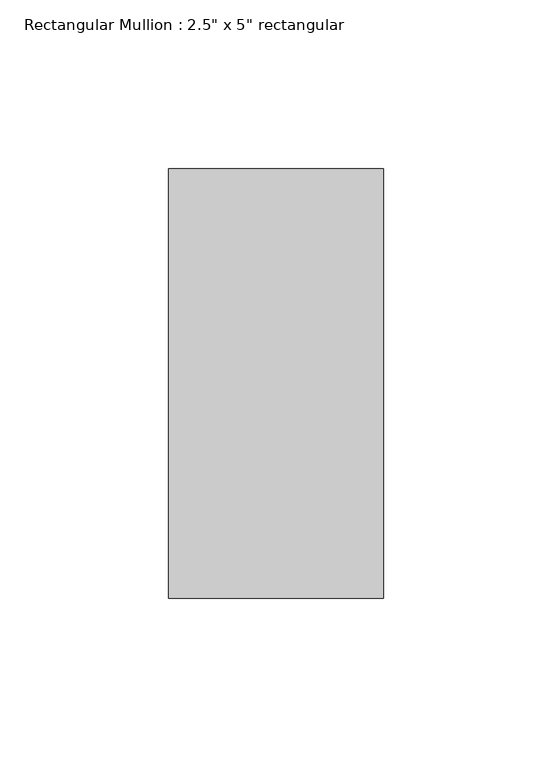
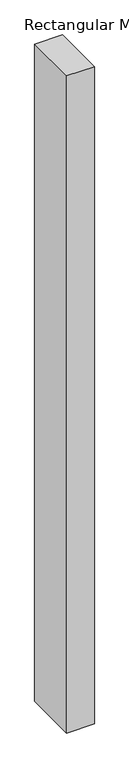
"""IFC4 building model written with IfcOpenShell, lengths in millimetres: member geometry."""

from ifc_helpers import new_model, si_unit, frame, origin, place, context, project, spatial, polyline, outline, extrude, source, transform, mapped, element, save


def member_87430b41(model_context):
    return source(origin(), model_context, "Body", "SweptSolid", [
        extrude(outline(polyline([(0.0, 63.5), (0.0, -63.5), (-63.5, -63.5), (-63.5, 63.5), (0.0, 63.5)])), frame((0.0, 0.0, -1593.034917), z_axis=(0.0, 0.0, 1.0), x_axis=(1.0, 0.0, 0.0)), (0.0, 0.0, 1.0), 1593.034917),
    ])


if __name__ == "__main__":
    model = new_model("IFC4")
    model_context = context("Model", 3, world=origin())
    ifc_project = project(units=[si_unit("LENGTHUNIT", "METRE", prefix="MILLI")], contexts=[model_context])
    site = spatial("IfcSite", under=ifc_project)
    building = spatial("IfcBuilding", under=site)
    placement = place(None, origin())
    member_shape = member_87430b41(model_context)
    element("IfcMember", 1, ObjectType="Rectangular Mullion : 2.5\" x 5\" rectangular", at=placement, inside=building, context=model_context, shape_type="MappedRepresentation", body=[
        mapped(member_shape, transform((0.0, 0.0, 0.0), x_axis=(1.0, 0.0, 0.0), y_axis=(0.0, 1.0, 0.0), z_axis=(0.0, 0.0, 1.0))),
    ])
    save(model, "model.ifc")

# Revit data of these elements
# Type "Rectangular Mullion : 2.5\" x 5\" rectangular"
#   built-in parameter 1007304 = 0.416667 (stored number, unit not read)
#   built-in parameter 1007301 = 0.104167 (stored number, unit not read)
#   built-in parameter 1007300 = 0.104167 (stored number, unit not read)
# Element 1 (IfcMember, "Rectangular Mullion : 2.5\" x 5\" rectangular")
#   Materials on its faces: "Aluminum"
# Materials
#   "Aluminum": class "Metal", colour RGB 247 247 247, transparency 0, Description = "Aluminum 6061", Cost = 0
